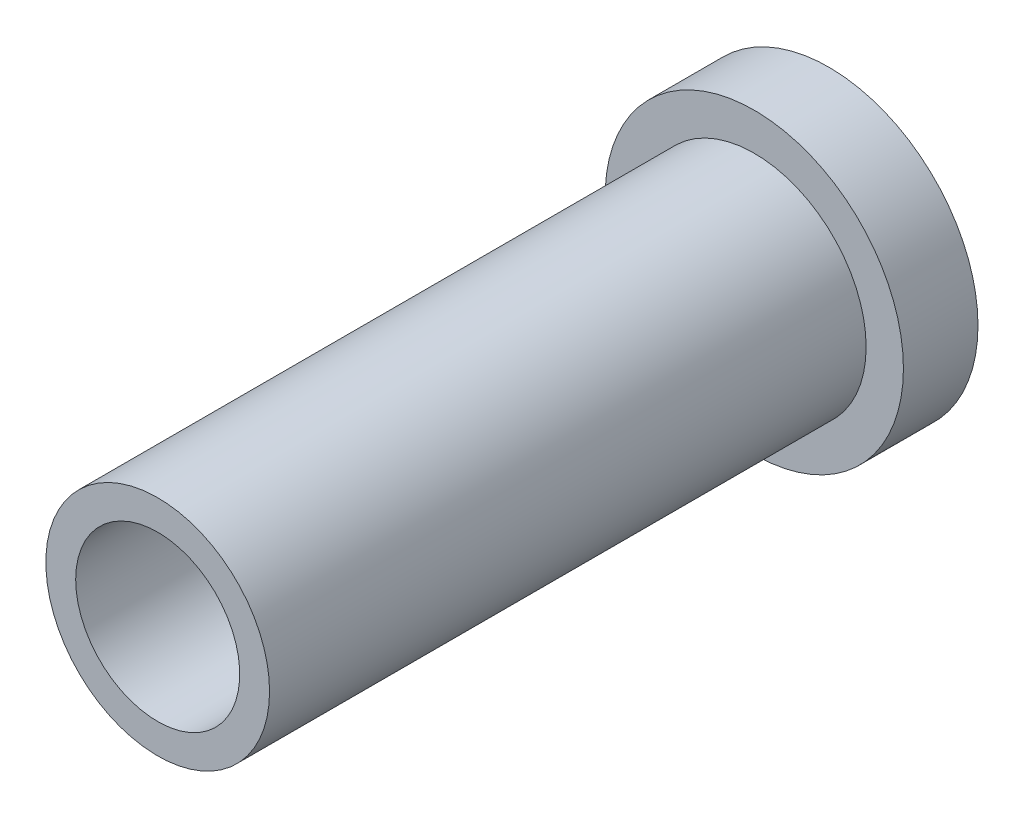
SolidWorks part; units mm, degrees
material "Plain Carbon Steel"
ref_plane "Front Plane" through (0, 0, 0) normal (0, 0, 1) x (1, 0, 0)
ref_plane "Top Plane" through (0, 0, 0) normal (0, 1, 0) x (1, 0, 0)
ref_plane "Right Plane" through (0, 0, 0) normal (1, 0, 0) x (0, 0, -1)
sketch "Flange Profile Ø20" plane through (0, 0, 0) normal (0, 0, 1) x (1, 0, 0)
  circle A0 centre (0, 0) radius 10
  dimension "D1" = 20
extrude "Flange Ø20x5" add sketch "Flange Profile Ø20" along normal blind 5
sketch "Shank Profile Ø15" plane through (0, 0, 5) normal (0, 0, 1) x (1, 0, 0)
  circle A0 centre (0, 0) radius 7.5
  dimension "D1" = 15
extrude "Shank Ø15x40" add sketch "Shank Profile Ø15" along normal blind 40
sketch "Bore Profile Ø11" plane through (0, 0, 0) normal (0, 0, -1) x (-1, 0, 0)
  circle A0 centre (0, 0) radius 5.5
  dimension "D1" = 11
extrude "Bore Ø11 Through" cut sketch "Bore Profile Ø11" against normal through all
